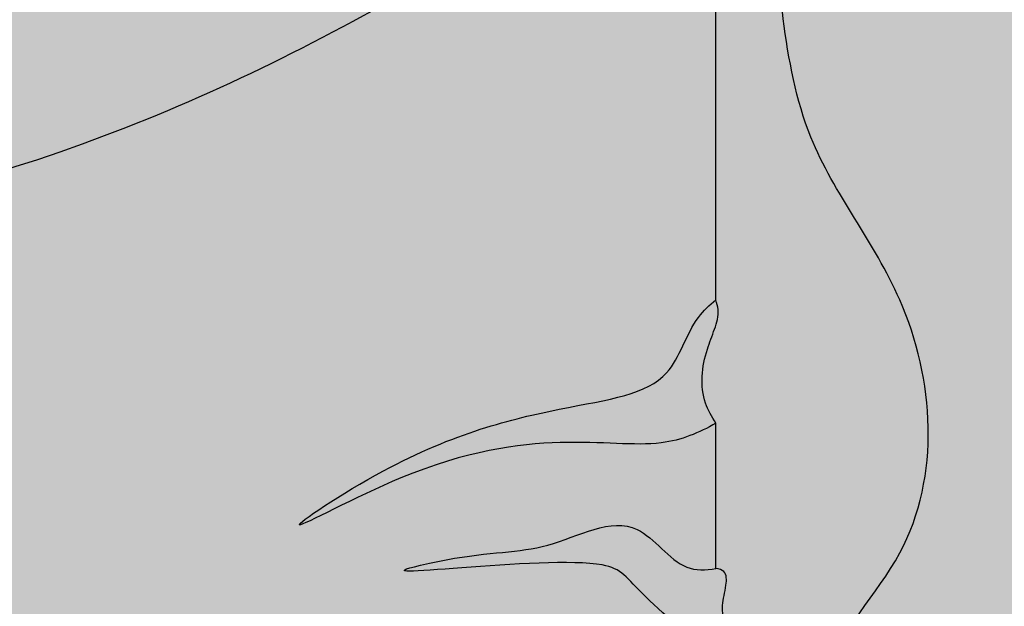
# Model space of a CAD drawing. Units: inches. Extents: x 1704 to 6393, y -157 to 1172.
# Tile 34 of 122: x 2548.79 to 2563.15, y 139.14 to 147.7. Entities that reach past the tile are written whole.
import ezdxf

# ---------------------------------------------------------------- set-up
doc = ezdxf.new("R2010")
doc.units = ezdxf.units.IN
doc.header["$MEASUREMENT"] = 0
for name, color, linetype, lineweight in [('A-ANNO-DIMS', 7, 'Continuous', 13), ('A-FURN', 8, 'Continuous', 18), ('estofado', 7, 'Continuous', 25)]:
    doc.layers.add(name, color=color, linetype=linetype, lineweight=lineweight)
doc.layers.add('A-FLOR-PATT', color=7, linetype='Continuous', lineweight=13, true_color=0xf2f2f2)
doc.styles.get("Standard").update_dxf_attribs({"font": 'arial.ttf'})
doc.dimstyles.get("Standard").update_dxf_attribs({"dimtxt": 6, "dimasz": 2, "dimexe": 0.18, "dimexo": 0.0625, "dimgap": 0.09, "dimtad": 0, "dimtih": 1, "dimtoh": 1, "dimdec": 1, "dimzin": 0, "dimdsep": 46, "dimlunit": 3, "dimtxsty": 'Standard', "dimblk": 'ARCHTICK', "dimcen": 0.09, "dimadec": 0, "dimazin": 0, "dimtfac": 1, "dimtdec": 1, "dimtofl": 0, "dimtmove": 0, "dimatfit": 3, "dimfxl": 1, "dimtolj": 1, "dimtzin": 0, "dimarcsym": 0})

# ---------------------------------------------------------------- blocks, each defined once
blk = doc.blocks.new('Cama Box Regencia LOLA')
at = {"layer": 'estofado', "ltscale": 0.2}
h = blk.add_hatch(color=256, dxfattribs=at)
h.dxf.hatch_style = 1
h.set_gradient(color1=(240, 232, 219), color2=(213, 190, 154), one_color=1, tint=0.7200000286102295)
edge = h.paths.add_edge_path()
edge.add_line((-0.8000000000000682, -0.1548023628405417), (-0.863597199697665, -0.2293271111754507))
edge.add_spline(control_points=[(-0.8635971996977787, -0.2293271111754507), (-0.8537222782123308, -0.258285373872468), (-0.8269013755602826, -0.3369378214810581), (-0.8674912876567759, -0.4595932758330151), (-0.8253488717912205, -0.6001498518888299), (-0.8771423076391329, -0.7139760714239288), (-0.8243323781925938, -0.8129899320257435), (-0.885044987287756, -0.8716602542656914), (-0.879518062107536, -0.9542863467743244), (-0.8339551707063037, -1.008464155856984), (-0.8245672924600739, -1.059984630119799), (-0.8208601923470268, -1.104655887174089), (-0.8073908324747662, -1.131238421004809), (-0.7999999999999546, -1.145824641594799)], knot_values=[0, 0, 0, 0, 0.0901802310564388, 0.2449351320798513, 0.3646438241986237, 0.5132330690395209, 0.5950634960661151, 0.646820388242338, 0.740988272125753, 0.8098674202588053, 0.8551784313864677, 0.8950360916221496, 0.9434986994854018, 0.9434986994854018, 0.9434986994854018, 0.9434986994854018], degree=3, periodic=0)
edge.add_line((-0.7999999999999546, -1.145824641594856), (-0.7999999999999546, -0.9571831923306604))
edge.add_spline(control_points=[(-0.8000000000001818, -0.9571831923294098), (-0.8003674620557603, -0.9560020588672273), (-0.8014778173377408, -0.9524330433489467), (-0.799534669348418, -0.9460450666617248), (-0.7963405736333016, -0.9382358308520792), (-0.7944188048602429, -0.9289040147384638), (-0.7953122817383474, -0.9190683391483389), (-0.7985341887020923, -0.9137677522519994), (-0.7999999999999546, -0.911356242470788)], knot_values=[0, 0, 0, 0, 0.0036609130031785, 0.0110621328900358, 0.0190316076023675, 0.0292873612819121, 0.0393286152452009, 0.0477100398955968, 0.0477100398955968, 0.0477100398955968, 0.0477100398955968], degree=3, periodic=0)
edge.add_line((-0.8000000000000682, -0.9113562424705037), (-0.7999999999999546, -0.8573491405791173))
edge.add_spline(control_points=[(-0.7999999999999546, -0.8573491405791173), (-0.8011509914009592, -0.8570771933481751), (-0.804102924754261, -0.8563797336621519), (-0.8039036519178353, -0.8498286502876908), (-0.8010279369466388, -0.8413595542568258), (-0.805623441450507, -0.8302818657685406), (-0.801318481758244, -0.8238273834048186), (-0.7999999999999546, -0.8218505664625013)], knot_values=[0, 0, 0, 0, 0.0032305881034183, 0.0082854491905874, 0.015951437769388, 0.0315866871777379, 0.0384893971878813, 0.0384893971878813, 0.0384893971878813, 0.0384893971878813], degree=3, periodic=0)
edge.add_line((-0.7999999999999546, -0.821850566462558), (-0.7999999999999546, -0.7800193173444541))
edge.add_spline(control_points=[(-0.7999999999999546, -0.7800193173443404), (-0.7985416092056994, -0.7788853679199974), (-0.7956241855360986, -0.7766169698310819), (-0.7929439183725436, -0.7707329795046576), (-0.7969680334608711, -0.7644035258254576), (-0.7912681985083055, -0.7566015403456845), (-0.7963938877088595, -0.7483952775559715), (-0.798936373489596, -0.7431699116222604), (-0.799999999999841, -0.7409839258539251)], knot_values=[0, 0, 0, 0, 0.0055481279082489, 0.0110986984731684, 0.0174746050947868, 0.0251556172852474, 0.035519246289823, 0.0429729849735991, 0.0429729849735991, 0.0429729849735991, 0.0429729849735991], degree=3, periodic=0)
edge.add_line((-0.7999999999999546, -0.740983925853584), (-0.8000000000000682, -0.1548023628405417))
h = blk.add_hatch(color=256, dxfattribs=at)
h.dxf.hatch_style = 1
h.set_gradient(color1=(240, 232, 219), color2=(213, 190, 154), one_color=1, tint=0.7200000286102295, name='CURVED')
edge = h.paths.add_edge_path()
edge.add_spline(control_points=[(0.343533776195045, -0.8455058148597345), (0.2879313990920309, -0.8167160606696484), (0.2054770794474052, -0.7744470032542381), (0.0954193394759386, -0.7742416952675626), (-0.0885363502328574, -0.7276964167006668), (0.2428192566063672, -0.7672518992321216), (0.345087521536243, -0.8076697826234067), (0.3825206986321063, -0.8228555492498799)], knot_values=[0.0056315103357428, 0.0056315103357428, 0.0056315103357428, 0.0056315103357428, 0.1860138916206105, 0.2660015162584448, 0.3570871810327863, 0.5963901805690979, 0.739731738908988, 0.739731738908988, 0.739731738908988, 0.739731738908988], degree=3, periodic=0)
edge.add_spline(control_points=[(0.3825206986325611, -0.8228555492497662), (0.3974221570828149, -0.8135511441712424), (0.4121061736600496, -0.8037181558521524), (0.4266849906532571, -0.7937075488799225)], knot_values=[1.358237767273279, 1.358237767273279, 1.358237767273279, 1.358237767273279, 1.409915662372559, 1.409915662372559, 1.409915662372559, 1.409915662372559], degree=3, periodic=0)
edge.add_spline(control_points=[(0.4266849905698109, -0.7937075489369932), (0.3998777739682282, -0.7821381809783361), (0.3476761897024971, -0.7634757898491671), (0.2670618099601825, -0.7565375622627358), (0.0835725072796549, -0.7192994417154637), (0.288524529784695, -0.7446405493717521), (0.4247448861246994, -0.7759943071475277), (0.4449816270193879, -0.7810438091316882)], knot_values=[0.1043639306803623, 0.1043639306803623, 0.1043639306803623, 0.1043639306803623, 0.1896363068641149, 0.2696239315019491, 0.3607095962762907, 0.6000125958126024, 0.6446217338078729, 0.6446217338078729, 0.6446217338078729, 0.6446217338078729], degree=3, periodic=0)
edge.add_spline(control_points=[(0.4449816270197289, -0.7810438091316882), (0.5029779388527232, -0.7406836481117695), (0.5966687145296419, -0.6736247633211292), (0.7071737530245628, -0.6656573253703187), (0.7517012483331201, -0.6672238302253392)], knot_values=[1.43159032281798, 1.43159032281798, 1.43159032281798, 1.43159032281798, 1.63814180148235, 1.770695287284994, 1.770695287284994, 1.770695287284994, 1.770695287284994], degree=3, periodic=0)
edge.add_arc((0.7481853615017826, -0.767162003811734), 0.0999999999999888, 58.7920033978138, 87.98512997550938, ccw=False)
edge.add_line((0.8000000000000682, -0.6816328085782289), (0.8000000000000682, -0.154802362840428))
edge.add_line((0.8000000000000682, -0.154802362840428), (-0.7999999999999546, -0.154802362840428))
edge.add_line((-0.7999999999999546, -0.154802362840428), (-0.8000000000000682, -0.7409839258539819))
edge.add_spline(control_points=[(-0.799999999999841, -0.7409839258539251), (-0.7846451382113174, -0.74846387981205), (-0.7568940913494089, -0.7651582159765554), (-0.7559936909002545, -0.8096905380045313), (-0.7049413305308008, -0.8142555457367848), (-0.7013836936888538, -0.8139988647640733)], knot_values=[0.0122267587020837, 0.0122267587020837, 0.0122267587020837, 0.0122267587020837, 0.0594720782072034, 0.1062176618094138, 0.134458043575382, 0.134458043575382, 0.134458043575382, 0.134458043575382], degree=3, periodic=0)
edge.add_spline(control_points=[(-0.7013836936890812, -0.8139988647637892), (-0.6428309483887916, -0.8132695376718857), (-0.532520673001045, -0.8118955240036598), (-0.2390712668254764, -0.6717984706609172), (-0.3892411364554391, -0.7557901092520752), (-0.4591093260188473, -0.8070101468627512), (-0.5571511178645779, -0.795652750469742), (-0.608497950975675, -0.8409486634728295), (-0.6632498050151981, -0.8266781836207997), (-0.6991149398675134, -0.8254126024436914), (-0.719552182989446, -0.8246914287938125)], knot_values=[0, 0, 0, 0, 0.2187005959148062, 0.4120203559900679, 0.4786136596093368, 0.6046444033330721, 0.6969970394608519, 0.7456449795902803, 0.7925683322559657, 0.8547274388453192, 0.8547274388453192, 0.8547274388453192, 0.8547274388453192], degree=3, periodic=0)
edge.add_spline(control_points=[(-0.7195521829781911, -0.824691428792164), (-0.7293124663336812, -0.8248308281530967), (-0.7545977292818407, -0.8216412233076653), (-0.7742556984202338, -0.794819860189591), (-0.7939222919129634, -0.7820064600295497), (-0.799999999999841, -0.7800193173443404)], knot_values=[0.1564883932805935, 0.1564883932805935, 0.1564883932805935, 0.1564883932805935, 0.184397548386913, 0.2313764834161266, 0.2505984550882281, 0.2505984550882281, 0.2505984550882281, 0.2505984550882281], degree=3, periodic=0)
edge.add_line((-0.8000000000000682, -0.7800193173444541), (-0.7999999999999546, -0.8218505664627286))
edge.add_spline(control_points=[(-0.7999999999999546, -0.8218505664625013), (-0.7938082505512511, -0.8290217081292894), (-0.7673857405620766, -0.8512914803976059), (-0.7619109683460011, -0.8661369353891359), (-0.6555700939965164, -0.8510070218793543), (-0.7139793977868294, -0.8637526923380391), (-0.7379026254519659, -0.8623504601624176), (-0.7688129786438367, -0.8813042143888196), (-0.7854260296310259, -0.8561610219318254), (-0.7961930533253962, -0.8566031243811949), (-0.7999999999999546, -0.8573491405791173)], knot_values=[0.0595743221876141, 0.0595743221876141, 0.0595743221876141, 0.0595743221876141, 0.08075289116965, 0.1037414994169835, 0.1697200936249022, 0.1760361327243865, 0.2071371586311508, 0.2404744334261798, 0.2623408547027293, 0.2736604507987723, 0.2736604507987723, 0.2736604507987723, 0.2736604507987723], degree=3, periodic=0)
edge.add_line((-0.7999999999999546, -0.8573491405791173), (-0.8000000000000682, -0.9113562424721521))
edge.add_spline(control_points=[(-0.8000000000000682, -0.9113562424720385), (-0.7937204054647964, -0.9077594990848183), (-0.7710343135782978, -0.8978798065321029), (-0.7213062468074442, -0.9144666877443228), (-0.6268586829058905, -0.862430497409548), (-0.6896594748232019, -0.9045634991654196), (-0.7483442493064559, -0.9189273406958591), (-0.7835301183422417, -0.922920432793262), (-0.7896301351460125, -0.9477657000142585), (-0.7975786973822779, -0.955260590410262), (-0.8000000000001818, -0.9571831923294098)], knot_values=[0.0138560263374175, 0.0138560263374175, 0.0138560263374175, 0.0138560263374175, 0.0348737775836104, 0.0888666909546002, 0.1078792274429341, 0.1267378491223226, 0.1587140219647659, 0.1937574699451985, 0.2174867851300671, 0.2267221218327879, 0.2267221218327879, 0.2267221218327879, 0.2267221218327879], degree=3, periodic=0)
edge.add_line((-0.7999999999999546, -0.957183192329296), (-0.7999999999999546, -1.145824641594742))
edge.add_spline(control_points=[(-0.8000000000002955, -1.145824641594913), (-0.7271039467997298, -1.094596787649038), (-0.4885706936571524, -0.9465888221489535), (-0.0701640902225336, -0.9707493165000187), (0.237911901821235, -0.902164522332157), (0.3435337762145991, -0.845505814843193)], knot_values=[0.1168958193629841, 0.1168958193629841, 0.1168958193629841, 0.1168958193629841, 0.3797203297758731, 0.9577018633805092, 1.31379338443587, 1.31379338443587, 1.31379338443587, 1.31379338443587], degree=3, periodic=0)
h.paths.add_polyline_path([(-0.6766340706021765, -0.6101327540145576, -0.3575266660906883), (-0.7312746368313583, -0.6354535276154252, -0.3575266660894137), (-0.7059538632299791, -0.5808129613865844, -0.1647847126465284), (-0.7059538632300928, -0.2676124402649407, -0.3575266660890756), (-0.7312746368312446, -0.2129718740360431, -0.3575266660908716), (-0.6766340706020629, -0.2382926476369676, -0.0925607043966334), (-0.1295169377724505, -0.2382926476369107, -0.3575266660898965), (-0.0748763715433825, -0.2129718740360431, -0.3575266660894428), (-0.1001971451446479, -0.2676124402649407, -0.1647847126465285), (-0.1001971451445343, -0.5808129613865844, -0.3575266660890756), (-0.0748763715433825, -0.6354535276154821, -0.3575266660898962), (-0.1295169377724505, -0.6101327540146145, -0.0925607043966531)], flags=16)
h.paths.add_polyline_path([(0.0748763715433825, -0.6354535276157094, -0.3575266660910266), (0.1001971451446479, -0.5808129613865844, -0.1647847126465284), (0.1001971451445343, -0.2676124402649407, -0.3575266660890757), (0.0748763715433825, -0.2129718740360431, -0.3575266660898962), (0.1295169377724505, -0.2382926476369107, -0.0925607043966334), (0.6766340706020629, -0.2382926476369676, -0.3575266660908718), (0.7312746368312446, -0.2129718740360431, -0.3575266660894425), (0.7059538632299791, -0.2676124402649407, -0.1647847126465283), (0.7059538632300928, -0.5808129613865844, -0.3575266660890756), (0.7312746368312446, -0.6354535276154821, -0.3575266660908716), (0.6766340706020629, -0.6101327540145576, -0.0925607043966335), (0.1295169377724505, -0.6101327540146145, -0.3575266660906303)], flags=16)
h = blk.add_hatch(color=256, dxfattribs=at)
h.dxf.hatch_style = 1
h.set_gradient(color1=(206, 178, 131), color2=(227, 212, 186), one_color=1, tint=0.8100000023841857, name='CYLINDER')
edge = h.paths.add_edge_path()
edge.add_arc((0.7481853614966667, -0.7671620038115634), 0.0999999999999888, 342.0511336145294, 447.9851299725766)
edge.add_spline(control_points=[(0.7517012483331201, -0.6672238302253392), (0.7071737530245628, -0.6656573253703187), (0.5966687145298692, -0.6736247633211292), (0.5029779388527232, -0.7406836481117125), (0.4449816270195015, -0.7810438091316314)], knot_values=[1.431590322817835, 1.431590322817835, 1.431590322817835, 1.431590322817835, 1.564143808620479, 1.770695287284994, 1.770695287284994, 1.770695287284994, 1.770695287284994], degree=3, periodic=0)
edge.add_spline(control_points=[(0.4449816270195015, -0.7810438091316314), (0.4388957332065502, -0.7852790380018178), (0.4327996148541616, -0.7895089160493285), (0.4266849906533708, -0.7937075488798087)], knot_values=[1.409915662372814, 1.409915662372814, 1.409915662372814, 1.409915662372814, 1.431590322817835, 1.431590322817835, 1.431590322817835, 1.431590322817835], degree=3, periodic=0)
edge.add_spline(control_points=[(0.4266849906533708, -0.7937075488798087), (0.4121061736600496, -0.8037181558521524), (0.3974221570825875, -0.8135511441712991), (0.38252069863222, -0.8228555492498799)], knot_values=[1.358237767273037, 1.358237767273037, 1.358237767273037, 1.358237767273037, 1.409915662372815, 1.409915662372815, 1.409915662372815, 1.409915662372815], degree=3, periodic=0)
edge.add_line((0.3825206986330158, -0.8228555492493114), (0.343533776286904, -0.8455058148063584))
edge.add_spline(control_points=[(0.3435337761924302, -0.8455058148550165), (0.2379119018048641, -0.902164522335795), (-0.0701640902311738, -0.9707493164995071), (-0.4885706936571524, -0.9465888221488967), (-0.7271039467997298, -1.094596787649038), (-0.8000000000000682, -1.145824641594742)], knot_values=[0.1168958193630798, 0.1168958193630798, 0.1168958193630798, 0.1168958193630798, 0.472987340393773, 1.050968873998409, 1.313793384411202, 1.313793384411202, 1.313793384411202, 1.313793384411202], degree=3, periodic=0)
edge.add_spline(control_points=[(-0.8000000000000682, -1.145824641594742), (-0.8038896190357718, -1.14855807951244), (-0.8077744942224853, -1.151305646504738), (-0.8116551946761774, -1.154065647517199)], knot_values=[0.1028719158199011, 0.1028719158199011, 0.1028719158199011, 0.1028719158199011, 0.1168958193630799, 0.1168958193630799, 0.1168958193630799, 0.1168958193630799], degree=3, periodic=0)
edge.add_arc((-0.7536973518524519, -1.235557294053705), 0.1000000000000352, 125.4208969883762, 169.6981795679068)
edge.add_spline(control_points=[(-0.852085287466366, -1.217673946333093), (-0.8521399740518518, -1.217974812833915), (-0.8565649010855622, -1.242328483616745), (-0.8662697220019026, -1.297321141147904), (-0.8487158298532904, -1.34896742172242), (-0.8348745804664758, -1.381844109035796)], knot_values=[0.3128349436863077, 0.3128349436863077, 0.3128349436863077, 0.3128349436863077, 0.3137509534211996, 0.386958004641742, 0.4759027329026081, 0.4759027329026081, 0.4759027329026081, 0.4759027329026081], degree=3, periodic=0)
edge.add_spline(control_points=[(-0.8348745804664758, -1.38184410903591), (-0.8226532004149476, -1.367823298399059), (-0.8056354908857201, -1.352141651537124), (-0.7460155199962628, -1.32170802000337)], knot_values=[0.0062456970656236, 0.0062456970656236, 0.0062456970656236, 0.0062456970656236, 0.0554759259147193, 0.0554759259147193, 0.0554759259147193, 0.0554759259147193], degree=3, periodic=0)
edge.add_spline(control_points=[(-0.7460155200169539, -1.321708019985464), (-0.6188339616464873, -1.25080943574278), (-0.3488365122128698, -1.179158668568902), (0.0338148848931041, -1.279726484458706), (0.3977250465933366, -1.412092721352792), (0.6449024721503065, -1.106270719748692), (0.7873766543807506, -1.256744909425322), (0.8547271521993025, -1.327877176513538)], knot_values=[0.0991852523588446, 0.0991852523588446, 0.0991852523588446, 0.0991852523588446, 0.5236467270390676, 0.9270872950244264, 1.289918234564769, 1.564439021262726, 1.810554634340498, 1.810554634340498, 1.810554634340498, 1.810554634340498], degree=3, periodic=0)
edge.add_arc((0.5509678495186563, -1.223443291813453), 0.3212104454069235, 341.0267878798241, 383.7782184284114)
edge.add_arc((1.292676354991499, -0.9435407756057543), 0.4723459732861395, 162.0511336103901, 198.5657216587827, ccw=False)
h = blk.add_hatch(color=256, dxfattribs=at)
h.dxf.hatch_style = 1
h.set_gradient(color1=(240, 232, 219), color2=(137, 106, 57), one_color=1, tint=0.3799999952316284, name='CURVED')
edge = h.paths.add_edge_path()
edge.add_spline(control_points=[(-0.7999999999999546, -0.8573491405791173), (-0.7961930533253962, -0.8566031243811949), (-0.7854260296310259, -0.8561610219318254), (-0.7688129786438367, -0.8813042143888196), (-0.7379026254519659, -0.8623504601624176), (-0.7139793977868294, -0.8637526923380391), (-0.6555700939965164, -0.8510070218793543), (-0.7619109683460011, -0.8661369353891359), (-0.7673857405620766, -0.8512914803976059), (-0.7938082505512511, -0.8290217081292894), (-0.7999999999999546, -0.8218505664625013)], knot_values=[0.0595743221876141, 0.0595743221876141, 0.0595743221876141, 0.0595743221876141, 0.0708939182836571, 0.0927603395602066, 0.1260976143552356, 0.1571986402619999, 0.1635146793614841, 0.2294932735694029, 0.2524818818167364, 0.2736604507987723, 0.2736604507987723, 0.2736604507987723, 0.2736604507987723], degree=3, periodic=0)
edge.add_spline(control_points=[(-0.7999999999999546, -0.8218505664625013), (-0.801318481758244, -0.8238273834048186), (-0.805623441450507, -0.8302818657685406), (-0.8010279369466388, -0.8413595542568258), (-0.8039036519178353, -0.8498286502876908), (-0.804102924754261, -0.8563797336621519), (-0.8011509914009592, -0.8570771933481751), (-0.7999999999999546, -0.8573491405791173)], knot_values=[0, 0, 0, 0, 0.0069027100101435, 0.0225379594184934, 0.030203947997294, 0.0352588090844631, 0.0384893971878813, 0.0384893971878813, 0.0384893971878813, 0.0384893971878813], degree=3, periodic=0)
h = blk.add_hatch(color=256, dxfattribs=at)
h.dxf.hatch_style = 1
h.set_gradient(color1=(240, 232, 219), color2=(137, 106, 57), one_color=1, tint=0.3799999952316284, name='CURVED')
edge = h.paths.add_edge_path()
edge.add_spline(control_points=[(-0.8000000000001818, -0.9571831923294098), (-0.7975786973822779, -0.955260590410262), (-0.7896301351460125, -0.9477657000142585), (-0.7835301183422417, -0.922920432793262), (-0.7483442493064559, -0.9189273406958591), (-0.6896594748232019, -0.9045634991654196), (-0.6268586829058905, -0.862430497409548), (-0.7213062468074442, -0.9144666877443228), (-0.7710343135782978, -0.8978798065321029), (-0.7937204054647964, -0.9077594990848183), (-0.8000000000000682, -0.9113562424720385)], knot_values=[0.0138560263374175, 0.0138560263374175, 0.0138560263374175, 0.0138560263374175, 0.0230913630401383, 0.0468206782250069, 0.0818641262054395, 0.1138402990478828, 0.1326989207272713, 0.1517114572156053, 0.205704370586595, 0.2267221218327879, 0.2267221218327879, 0.2267221218327879, 0.2267221218327879], degree=3, periodic=0)
edge.add_spline(control_points=[(-0.7999999999999546, -0.911356242470788), (-0.7985341887020923, -0.9137677522519994), (-0.7953122817383474, -0.9190683391483389), (-0.7944188048602429, -0.9289040147384638), (-0.7963405736333016, -0.9382358308520792), (-0.799534669348418, -0.9460450666617248), (-0.8014778173377408, -0.9524330433489467), (-0.8003674620557603, -0.9560020588672273), (-0.8000000000001818, -0.9571831923294098)], knot_values=[0, 0, 0, 0, 0.008381424650396, 0.0184226786136847, 0.0286784322932294, 0.0366479070055611, 0.0440491268924183, 0.0477100398955968, 0.0477100398955968, 0.0477100398955968, 0.0477100398955968], degree=3, periodic=0)
for points in [[(-0.7999999999999546, -0.8573491405790605), (-0.7999999999999546, -0.9113562424710153)], [(-0.7999999999999546, -0.9571831923292393), (-0.7999999999999546, -1.145824641594799)]]:
    blk.add_lwpolyline(points, dxfattribs=at)
for points, knots in [([(-0.8635971996977787, -0.2293271111754507), (-0.8537222782123597, -0.2582853738724713), (-0.8269013755602529, -0.3369378214810687), (-0.8674912876567628, -0.459593275832977), (-0.8253488717912105, -0.6001498518888299), (-0.8771423076387755, -0.7139760714238776), (-0.824332378192706, -0.8129899320257793), (-0.8850449872876955, -0.8716602542656513), (-0.8795180621076731, -0.9542863467744586), (-0.8339551707061605, -1.008464155856879), (-0.8245672924602526, -1.059984630119836), (-0.820860192346876, -1.104655887174075), (-0.8073908324747767, -1.131238421004865), (-0.7999999999999546, -1.145824641594799)], [0, 0, 0, 0, 0.0901802310564388, 0.2449351320798513, 0.3646438241986237, 0.5132330690395209, 0.5950634960661151, 0.646820388242338, 0.740988272125753, 0.8098674202588053, 0.8551784313864677, 0.8950360916221496, 0.9434986994854018, 0.9434986994854018, 0.9434986994854018, 0.9434986994854018]), ([(-0.7999999999999546, -0.8218505664625013), (-0.8013184817582112, -0.8238273834047737), (-0.8056234414505565, -0.8302818657685486), (-0.8010279369466333, -0.8413595542568746), (-0.8039036519179351, -0.8498286502876482), (-0.80410292475424, -0.8563797336621606), (-0.8011509914010776, -0.857077193348196), (-0.7999999999999546, -0.8573491405791173)], [0, 0, 0, 0, 0.0069027100101435, 0.0225379594184934, 0.030203947997294, 0.0352588090844631, 0.0384893971878813, 0.0384893971878813, 0.0384893971878813, 0.0384893971878813]), ([(-0.7999999999999546, -0.8218505664625013), (-0.7938082505512511, -0.8290217081292894), (-0.7673857405620766, -0.8512914803976059), (-0.7619109683460011, -0.8661369353891359), (-0.6555700939965164, -0.8510070218793543), (-0.7139793977868294, -0.8637526923380391), (-0.7379026254519659, -0.8623504601624176), (-0.7688129786438367, -0.8813042143888196), (-0.7854260296310259, -0.8561610219318254), (-0.7961930533253962, -0.8566031243811949), (-0.7999999999999546, -0.8573491405791173)], [0.0595743221876141, 0.0595743221876141, 0.0595743221876141, 0.0595743221876141, 0.08075289116965, 0.1037414994169835, 0.1697200936249022, 0.1760361327243865, 0.2071371586311508, 0.2404744334261798, 0.2623408547027293, 0.2736604507987723, 0.2736604507987723, 0.2736604507987723, 0.2736604507987723]), ([(-0.8116551946761774, -1.154065647517199), (-0.7350455857787211, -1.099579968801037), (-0.493473113061782, -0.9463057365681493), (-0.0701640902311738, -0.9707493164995071), (0.2379119018048641, -0.902164522335795), (0.3435337761924302, -0.8455058148550165)], [0.1028719158199011, 0.1028719158199011, 0.1028719158199011, 0.1028719158199011, 0.3797203297758731, 0.9577018633805092, 1.313793384411202, 1.313793384411202, 1.313793384411202, 1.313793384411202]), ([(-0.8000000000000682, -0.9113562424720385), (-0.7937204054647964, -0.9077594990848183), (-0.7710343135782978, -0.8978798065321029), (-0.7213062468074442, -0.9144666877443228), (-0.6268586829058905, -0.862430497409548), (-0.6896594748232019, -0.9045634991654196), (-0.7483442493064559, -0.9189273406958591), (-0.7835301183422417, -0.922920432793262), (-0.7896301351460125, -0.9477657000142585), (-0.7975786973822779, -0.955260590410262), (-0.8000000000001818, -0.9571831923294098)], [0.0138560263374175, 0.0138560263374175, 0.0138560263374175, 0.0138560263374175, 0.0348737775836104, 0.0888666909546002, 0.1078792274429341, 0.1267378491223226, 0.1587140219647659, 0.1937574699451985, 0.2174867851300671, 0.2267221218327879, 0.2267221218327879, 0.2267221218327879, 0.2267221218327879]), ([(-0.7999999999999546, -0.911356242470788), (-0.7985341887021342, -0.913767752252043), (-0.795312281738289, -0.9190683391482961), (-0.7944188048601522, -0.9289040147384582), (-0.7963405736334027, -0.9382358308520572), (-0.7995346693483358, -0.946045066661701), (-0.8014778173378848, -0.9524330433489994), (-0.800367462055735, -0.9560020588672482), (-0.8000000000001818, -0.9571831923294098)], [0, 0, 0, 0, 0.008381424650396, 0.0184226786136847, 0.0286784322932294, 0.0366479070055611, 0.0440491268924183, 0.0477100398955968, 0.0477100398955968, 0.0477100398955968, 0.0477100398955968])]:
    blk.add_open_spline(points, degree=3, knots=knots, dxfattribs=at)
blk = doc.blocks.new('_ArchTick')
at = {"color": 0, "linetype": 'ByBlock', "const_width": 0.15}
blk.add_lwpolyline([(-0.5, -0.5), (0.5, 0.5)], dxfattribs=at)
blk = doc.blocks.new('*D93')
at = {"layer": 'A-ANNO-DIMS', "color": 0, "lineweight": -2, "transparency": 16777216}
for p, q in [((2605.286074000001, 895.2129740000005), (1829.697551000002, 895.2129740000003)), ((1829.877551000002, 895.2129740000003), (1829.877551000002, 495.8664119263302)), ((1829.877551000002, 90.2129739999999), (1829.877551000002, 489.5595360736699)), ((2605.286074000001, 90.21297400000003), (1829.697551000002, 90.2129739999999))]:
    blk.add_line(p, q, dxfattribs=at)
at = {"layer": 'Defpoints', "color": 0, "lineweight": -3, "transparency": 16777216}
for p in [(2605.348574000001, 895.2129740000005), (1829.877551000002, 90.2129739999999), (2605.348574000001, 90.21297400000003)]:
    blk.add_point(p, dxfattribs=at)
at = {"layer": 'A-ANNO-DIMS', "color": 0, "lineweight": -2, "transparency": 16777216, "xscale": 2, "yscale": 2, "zscale": 2}
for p, rotation in [((1829.877551000002, 895.2129740000003), 90), ((1829.877551000002, 90.2129739999999), 270)]:
    blk.add_blockref('_ArchTick', p, dxfattribs=dict(at, rotation=rotation))
at = {"layer": 'A-ANNO-DIMS', "color": 0, "transparency": 16777216, "insert": (1829.877551000001, 492.7129739999994), "char_height": 6, "attachment_point": 5}
blk.add_mtext('\\A1;805', dxfattribs=at)

msp = doc.modelspace()

# ---------------------------------------------------------------- hatches: boundary and pattern name
at = {"layer": 'A-FLOR-PATT', "transparency": 33554528}
h = msp.add_hatch(color=256, dxfattribs=at)
h.dxf.hatch_style = 1
h.paths.add_polyline_path([(2325.348574056059, 863.2129735309796), (2325.348574056059, 887.2129735309796), (2263.348574056059, 887.2129735309796), (2167.348574056059, 887.2129735309794), (2081.348574056061, 887.2129735309792), (2081.348574056061, 719.2129735309785), (2277.348574056059, 719.2129735309787), (2277.348574056059, 711.2129735309788), (2277.348574056059, 372.212973530979), (2349.348574056059, 372.212973530979), (2381.348574056059, 372.2129735309789), (2381.348574056059, 364.2129735309789), (2353.348574056059, 364.2129735309789), (2353.348574056059, 270.2129735309788), (2381.348574056059, 270.2129735309788), (2381.348574056059, 266.2129735309788), (2357.348574056059, 266.2129735309788), (2357.348574056059, 98.21297353097884), (2381.348574056059, 98.21297353097897), (2385.181056550604, 98.21297353097884), (2386.482186711948, 98.21297353097884), (2424.21496140017, 98.21297353097884), (2425.516091561514, 98.21297353097884), (2429.348574056059, 98.21297353097897), (2597.348574056059, 98.21297353097884), (2597.348574056059, 146.2129735309788), (2597.348574056059, 218.2129735309788), (2597.348574056059, 266.2129735309788), (2423.348574056059, 266.2129735309788), (2423.348574056059, 270.2129735309788), (2473.348574056059, 270.2129735309788), (2473.348574056059, 294.2129735309789), (2477.348574056059, 294.2129735309789), (2477.348574056059, 270.2129735309788), (2547.348574056059, 270.2129735309788), (2547.348574056059, 364.2129735309788), (2477.348574056059, 364.2129735309788), (2477.348574056059, 318.2129735309788), (2473.348574056059, 318.2129735309787), (2473.348574056059, 364.2129735309789), (2423.348574056059, 364.2129735309788), (2423.348574056059, 372.2129735309788), (2469.348574056059, 372.2129735309788), (2469.348574056059, 459.2129735309789), (2469.348574056059, 538.2129735309788), (2350.348574056059, 538.2129735309788), (2350.348574056059, 565.7129735309788), (2358.348574056059, 565.7129735309788), (2358.348574056059, 545.2129735309788), (2420.348574056059, 545.2129735309788), (2420.348574056059, 610.2129735309788), (2358.348574056059, 610.2129735309788), (2358.348574056059, 589.7129735309788), (2350.348574056059, 589.7129735309788), (2350.348574056059, 615.2129735309788), (2425.348574056059, 615.2129735309788), (2425.348574056059, 607.2129735309788), (2425.348574056059, 546.2129735309788), (2469.348574056059, 546.2129735309788), (2514.34857405606, 546.212973530979), (2514.34857405606, 607.2129735309788), (2449.348574056059, 607.2129735309788), (2449.348574056059, 615.2129735309788), (2451.737974987759, 615.2129735309788), (2451.737974987759, 659.2129735309788), (2427.737974987759, 659.2129735309788), (2427.737974987759, 665.2129735309788), (2367.737974987758, 665.2129735309788), (2367.737974987758, 667.2129735309788), (2367.737974987758, 711.2129735309788), (2325.348574056059, 711.2129735309788), (2325.348574056059, 719.2129735309785), (2325.348574056059, 755.2129735309787), (2325.348574056059, 763.2129735309788)])
h.paths.add_polyline_path([(2233.85817000392, 822.532660166629, -0.1872470486944155), (2233.85817000392, 809.1396667958562), (2231.697030374885, 808.8044951349628, 0.0848927708004382), (2233.130501812631, 814.4858417746204), (2230.423974436808, 814.4858417746204, -0.1042581087707907), (2228.553363812687, 808.3129425443484), (2217.750790159711, 807.1555239386723, -0.2222222222222219), (2217.750790159711, 824.5168030238124), (2228.553363812687, 823.3593844181363, -0.1042581087707933), (2230.423974436808, 817.1864851878643), (2233.130501812631, 817.1864851878643, 0.08489277080044), (2231.697030374885, 822.8678318275219)], flags=16)
h.paths.add_polyline_path([(2213.621360876743, 833.1974425663823), (2213.621360876743, 798.4748843961024), (2156.047684459484, 798.4748843961034), (2156.047684459485, 833.1974425663813)], flags=16)
h.paths.add_polyline_path([(2203.931929661768, 848.0987249710489), (2205.089348267444, 837.2961513180724, -0.2222222222222264), (2187.728069182304, 837.2961513180724), (2188.88548778798, 848.0987249710485, -0.104258108770792), (2195.058387018252, 849.9693355951691), (2195.058387018252, 852.6758629709927, 0.084892770800438), (2189.377040378595, 851.2423915332469), (2189.712212039488, 853.4035311622828, -0.1872470486944166), (2203.105205410261, 853.4035311622828), (2203.440377071154, 851.2423915332469, 0.084892770800438), (2197.759030431496, 852.6758629709927), (2197.759030431496, 849.9693355951691, -0.1042581087707896)], flags=16)
h.paths.add_polyline_path([(2181.940976153924, 837.2961513180726, -0.2222222222222323), (2164.579697068783, 837.2961513180724), (2165.73711567446, 848.0987249710487, -0.1042581087707905), (2171.910014904732, 849.9693355951691), (2171.910014904732, 852.6758629709927, 0.0848927708004445), (2166.228668265074, 851.2423915332469), (2166.563839925967, 853.403531162283, -0.1872470486944096), (2179.95683329674, 853.4035311622828), (2180.292004957633, 851.2423915332465, 0.0848927708004458), (2174.610658317976, 852.6758629709927), (2174.610658317976, 849.9693355951691, -0.104258108770801), (2180.783557548248, 848.0987249710482)], flags=16)
h.paths.add_polyline_path([(2205.089348267444, 794.376175644412), (2203.931929661768, 783.5736019914364, -0.1042581087707934), (2197.759030431496, 781.7029913673155), (2197.759030431496, 778.9964639914921, 0.084892770800439), (2203.440377071154, 780.4299354292382), (2203.105205410261, 778.2687958002022, -0.1872470486944172), (2189.712212039488, 778.2687958002018), (2189.377040378595, 780.4299354292377, 0.0848927708004369), (2195.058387018252, 778.9964639914919), (2195.058387018252, 781.7029913673153, -0.1042581087707904), (2188.88548778798, 783.5736019914358), (2187.728069182304, 794.3761756444126, -0.2222222222222231)], flags=16)
h.paths.add_polyline_path([(2181.940976153924, 794.376175644412), (2180.783557548248, 783.5736019914364, -0.1042581087708008), (2174.610658317976, 781.7029913673153), (2174.610658317976, 778.9964639914921, 0.0848927708004458), (2180.292004957633, 780.4299354292382), (2179.95683329674, 778.268795800202, -0.1872470486944096), (2166.563839925967, 778.2687958002018), (2166.228668265074, 780.4299354292378, 0.0848927708004446), (2171.910014904732, 778.9964639914919), (2171.910014904732, 781.7029913673153, -0.1042581087707904), (2165.73711567446, 783.5736019914358), (2164.579697068783, 794.3761756444123, -0.2222222222222294)], flags=16)
h.paths.add_polyline_path([(2151.918255176517, 807.1555239386723), (2141.115681523541, 808.3129425443484, -0.1042581087707911), (2139.24507089942, 814.4858417746204), (2136.538543523597, 814.4858417746204, 0.08489277080044), (2137.972014961343, 808.8044951349626), (2135.810875332307, 809.1396667958562, -0.1872470486944109), (2135.810875332307, 822.5326601666285), (2137.972014961343, 822.8678318275221, 0.0848927708004416), (2136.538543523597, 817.1864851878643), (2139.24507089942, 817.1864851878643, -0.104258108770793), (2141.115681523541, 823.3593844181363), (2151.918255176517, 824.5168030238124, -0.2222222222222205)], flags=16)
h.paths.add_polyline_path([(2357.868011454448, 363.4102250290031), (2358.813881560335, 363.4102250290031, 0.7537604849588476)], flags=16)
h.paths.add_polyline_path([(2372.241054283868, 363.1167008961685), (2372.248110816919, 363.1167008961685), (2372.248110816919, 363.3425764997267), (2371.30224071103, 363.3425764997267), (2371.30224071103, 363.1392706554335, -1.360391292333951)], flags=16)
h.paths.add_polyline_path([(2371.309297244092, 272.7157694655011), (2371.30224071103, 272.7157694655011), (2371.30224071103, 272.4898938619428), (2372.248110816919, 272.4898938619428), (2372.248110816919, 272.6931997062759, -1.360391292393621)], flags=16)
h.paths.add_polyline_path([(2357.875067987504, 272.7157694655011), (2357.868011454452, 272.7157694655011), (2357.868011454452, 272.4898938619428), (2358.813881560341, 272.4898938619428), (2358.813881560341, 272.6931997062361, -1.360391292333948)], flags=16)
h.paths.add_polyline_path([(2353.768696905258, 363.0736921025416), (2376.347425366111, 363.0736921025416), (2376.347425366111, 272.7587782591281), (2353.768696905258, 272.7587782591281)], flags=16)
h.paths.add_polyline_path([(2354.772195947961, 362.0701930598379), (2375.343926323407, 362.0701930598379), (2375.343926323407, 273.7622773018316), (2354.772195947961, 273.7622773018318)], flags=0)
h.paths.add_polyline_path([(2357.868011454452, 363.3425764997267), (2358.813881560341, 363.3425764997266), (2358.813881560341, 363.1167008961684), (2357.868011454452, 363.1167008961684)], flags=16)
h.paths.add_polyline_path([(2359.287941640134, 359.1843485433627), (2359.287941640134, 360.0631949744305), (2370.828180631237, 360.0631949744362), (2370.828180631237, 359.1843485433769), (2374.332057422314, 359.1843485433812), (2374.332057422312, 358.4635369582513), (2372.835178716611, 358.4635369582524), (2372.835178716611, 357.5410357047662), (2374.332057422314, 357.5410357047678), (2374.332057422312, 356.8202241196381), (2372.835178716611, 356.820224119639), (2372.835178716611, 355.897722866153), (2374.332057422314, 355.8977228661546), (2374.332057422312, 355.1769112810248), (2372.835178716611, 355.1769112810259), (2372.835178716611, 354.2544100275397), (2374.332057422334, 354.2544100275415), (2374.332057422331, 353.5335984424117), (2372.835178716631, 353.5335984424126), (2372.835178716631, 352.6110971889265), (2374.332057422334, 352.6110971889282), (2374.332057422331, 351.8902856037984), (2372.835178716631, 351.8902856037993), (2372.835178716631, 350.9677843503132), (2374.332057422334, 350.967784350315), (2374.332057422331, 350.2469727651852), (2372.835178716631, 350.2469727651861), (2372.835178716631, 349.3244715117), (2374.332057422334, 349.3244715117017), (2374.332057422331, 348.603659926572), (2372.835178716631, 348.6036599265729), (2372.835178716631, 347.6811586730868), (2374.332057422334, 347.6811586730886), (2374.332057422331, 346.9603470879587), (2372.835178716631, 346.9603470879598), (2372.835178716631, 346.0378458344735), (2374.332057422334, 346.0378458344753), (2374.332057422331, 345.3170342493456), (2372.835178716631, 345.3170342493465), (2372.835178716631, 344.3945329958605), (2374.332057422334, 344.3945329958621), (2374.332057422331, 343.6737214107324), (2372.835178716631, 343.6737214107334), (2372.835178716631, 342.751220157247), (2374.332057422334, 342.7512201572489), (2374.332057422331, 342.0304085721191), (2372.835178716631, 342.03040857212), (2372.835178716631, 341.1079073186338), (2374.332057422334, 341.1079073186356), (2374.332057422331, 340.3870957335057), (2372.835178716631, 340.3870957335066), (2372.835178716631, 339.4645944800207), (2374.332057422334, 339.4645944800223), (2374.332057422331, 338.7437828948924), (2372.835178716648, 338.7437828948933), (2372.835178716648, 337.8212816414076), (2374.332057422334, 337.8212816414093), (2374.332057422331, 337.1004700562794), (2372.835178716648, 337.1004700562803), (2372.835178716648, 336.1779688027942), (2374.332057422334, 336.1779688027961), (2374.332057422331, 335.4571572176662), (2372.835178716648, 335.4571572176673), (2372.835178716648, 334.5346559641809), (2374.332057422334, 334.5346559641828), (2374.332057422331, 333.8138443790529), (2372.835178716648, 333.8138443790539), (2372.835178716648, 332.8913431255679), (2374.332057422334, 332.8913431255696), (2374.332057422331, 332.1705315404397), (2372.835178716648, 332.1705315404406), (2372.835178716648, 331.2480302869545), (2374.332057422334, 331.2480302869563), (2374.332057422331, 330.5272187018265), (2372.835178716648, 330.5272187018273), (2372.835178716648, 329.6047174483413), (2374.332057422334, 329.6047174483431), (2374.332057422331, 328.8839058632133), (2372.835178716648, 328.8839058632143), (2372.835178716648, 327.9614046097282), (2374.332057422334, 327.9614046097298), (2374.332057422331, 327.2405930246), (2372.835178716648, 327.2405930246009), (2372.835178716648, 326.3180917711149), (2374.332057422334, 326.3180917711167), (2374.332057422331, 325.5972801859869), (2372.835178716648, 325.5972801859877), (2372.835178716648, 324.6747789325016), (2374.332057422334, 324.6747789325034), (2374.332057422331, 323.9539673473736), (2372.835178716648, 323.9539673473746), (2372.835178716648, 323.0314660938884), (2374.332057422334, 323.0314660938901), (2374.332057422331, 322.3106545087603), (2372.835178716648, 322.3106545087613), (2372.835178716648, 321.3881532552753), (2374.332057422334, 321.388153255277), (2374.332057422331, 320.6673416701471), (2372.835178716648, 320.6673416701481), (2372.835178716648, 319.7448404166621), (2374.332057422334, 319.7448404166638), (2374.332057422331, 319.0240288315339), (2372.835178716648, 319.0240288315348), (2372.835178716648, 318.1015275780487), (2374.332057422334, 318.1015275780504), (2374.332057422331, 317.3807159929205), (2372.835178716648, 317.3807159929214), (2372.835178716648, 316.4582147394357), (2374.332057422334, 316.4582147394373), (2374.332057422331, 315.7374031543073), (2372.835178716648, 315.7374031543084), (2372.835178716648, 314.8149019008223), (2374.332057422334, 314.8149019008241), (2374.332057422331, 314.0940903156943), (2372.835178716648, 314.0940903156952), (2372.835178716648, 313.171589062209), (2374.332057422334, 313.1715890622108), (2374.332057422331, 312.450777477081), (2372.835178716648, 312.4507774770819), (2372.835178716648, 311.5282762235959), (2374.332057422334, 311.5282762235977), (2374.332057422331, 310.8074646384678), (2372.835178716648, 310.8074646384687), (2372.835178716648, 309.8849633849827), (2374.332057422334, 309.8849633849844), (2374.332057422331, 309.1641517998546), (2372.835178716648, 309.1641517998555), (2372.835178716648, 308.2416505463693), (2374.332057422334, 308.2416505463712), (2374.332057422331, 307.5208389612412), (2372.835178716648, 307.5208389612421), (2372.835178716648, 306.5983377077562), (2374.332057422334, 306.598337707758), (2374.332057422331, 305.8775261226281), (2372.835178716648, 305.8775261226289), (2372.835178716648, 304.955024869143), (2374.332057422334, 304.9550248691447), (2374.332057422331, 304.2342132840149), (2372.835178716648, 304.2342132840158), (2372.835178716648, 303.3117120305298), (2374.332057422334, 303.3117120305316), (2374.332057422331, 302.5909004454018), (2372.835178716648, 302.5909004454027), (2372.835178716648, 301.6683991919165), (2374.332057422334, 301.6683991919183), (2374.332057422331, 300.9475876067885), (2372.835178716648, 300.9475876067894), (2372.835178716648, 300.0250863533033), (2374.332057422334, 300.025086353305), (2374.332057422331, 299.3042747681752), (2372.835178716648, 299.3042747681761), (2372.835178716648, 298.3817735146902), (2374.332057422334, 298.3817735146919), (2374.332057422331, 297.6609619295621), (2372.835178716648, 297.6609619295629), (2372.835178716648, 296.7384606760769), (2374.332057422334, 296.7384606760786), (2374.332057422331, 296.0176490909488), (2372.835178716648, 296.0176490909498), (2372.835178716648, 295.0951478374636), (2374.332057422334, 295.0951478374653), (2374.332057422331, 294.3743362523355), (2372.835178716648, 294.3743362523364), (2372.835178716648, 293.4518349988504), (2374.332057422334, 293.4518349988522), (2374.332057422331, 292.7310234137224), (2372.835178716648, 292.7310234137233), (2372.835178716648, 291.8085221602371), (2374.332057422334, 291.8085221602389), (2374.332057422331, 291.0877105751091), (2372.835178716648, 291.08771057511), (2372.835178716648, 290.165209321624), (2374.332057422334, 290.1652093216256), (2374.332057422331, 289.4443977364957), (2372.835178716648, 289.4443977364966), (2372.835178716648, 288.5218964830108), (2374.332057422334, 288.5218964830125), (2374.332057422331, 287.8010848978827), (2372.835178716648, 287.8010848978836), (2372.835178716648, 286.8785836443975), (2374.332057422334, 286.8785836443993), (2374.332057422331, 286.1577720592695), (2372.835178716648, 286.1577720592703), (2372.835178716648, 285.2352708057842), (2374.332057422334, 285.2352708057861), (2374.332057422331, 284.5144592206562), (2372.835178716648, 284.514459220657), (2372.835178716648, 283.5919579671712), (2374.332057422334, 283.5919579671728), (2374.332057422331, 282.871146382043), (2372.835178716648, 282.8711463820439), (2372.835178716648, 281.9486451285579), (2374.332057422334, 281.9486451285596), (2374.332057422331, 281.2278335434298), (2372.835178716648, 281.2278335434307), (2372.835178716648, 280.3053322899446), (2374.332057422334, 280.3053322899464), (2374.332057422331, 279.5845207048164), (2372.835178716648, 279.5845207048174), (2372.835178716648, 278.6620194513314), (2374.332057422334, 278.6620194513331), (2374.332057422331, 277.9412078662033), (2372.835178716648, 277.9412078662043), (2372.835178716648, 277.0187066127184), (2374.332057422334, 277.0187066127201), (2374.332057422331, 276.29789502759), (2370.828180631244, 276.2978950275922), (2370.828180631244, 275.7692753872335), (2359.287941640128, 275.7692753872392), (2359.287941640128, 276.2978950275993), (2355.784064849037, 276.2978950276015), (2355.784064849037, 277.0187066126971), (2357.280943554723, 277.0187066126989), (2357.280943554723, 277.9412078662137), (2355.784064849037, 277.9412078662145), (2355.784064849037, 278.6620194513103), (2357.280943554723, 278.6620194513122), (2357.280943554723, 279.5845207048271), (2355.784064849037, 279.584520704828), (2355.784064849037, 280.3053322899236), (2357.280943554723, 280.3053322899253), (2357.280943554723, 281.2278335434403), (2355.784064849037, 281.2278335434412), (2355.784064849037, 281.9486451285369), (2357.280943554723, 281.9486451285387), (2357.280943554723, 282.8711463820535), (2355.784064849037, 282.8711463820543), (2355.784064849037, 283.5919579671501), (2357.280943554723, 283.591957967152), (2357.280943554723, 284.5144592206668), (2355.784064849037, 284.5144592206676), (2355.784064849037, 285.2352708057632), (2357.280943554723, 285.2352708057651), (2357.280943554723, 286.1577720592801), (2355.784064849037, 286.1577720592809), (2355.784064849037, 286.8785836443766), (2357.280943554723, 286.8785836443784), (2357.280943554723, 287.8010848978931), (2355.784064849037, 287.8010848978941), (2355.784064849037, 288.5218964829895), (2357.280943554723, 288.5218964829913), (2357.280943554723, 289.4443977365064), (2355.784064849037, 289.4443977365072), (2355.784064849037, 290.1652093216029), (2357.280943554723, 290.1652093216047), (2357.280943554723, 291.0877105751197), (2355.784064849037, 291.0877105751206), (2355.784064849037, 291.8085221602161), (2357.280943554723, 291.8085221602179), (2357.280943554723, 292.7310234137328), (2355.784064849037, 292.7310234137337), (2355.784064849037, 293.4518349988293), (2357.280943554723, 293.451834998831), (2357.280943554723, 294.3743362523461), (2355.784064849037, 294.3743362523469), (2355.784064849037, 295.0951478374426), (2357.280943554723, 295.0951478374445), (2357.280943554723, 296.0176490909594), (2355.784064849037, 296.0176490909601), (2355.784064849037, 296.7384606760557), (2357.280943554723, 296.7384606760575), (2357.280943554723, 297.6609619295724), (2355.784064849037, 297.6609619295734), (2355.784064849037, 298.3817735146691), (2357.280943554723, 298.3817735146709), (2357.280943554723, 299.3042747681858), (2355.784064849037, 299.3042747681866), (2355.784064849037, 300.0250863532823), (2357.280943554723, 300.0250863532841), (2357.280943554723, 300.9475876067989), (2355.784064849037, 300.9475876067997), (2355.784064849037, 301.6683991918954), (2357.280943554723, 301.6683991918973), (2357.280943554723, 302.5909004454123), (2355.784064849037, 302.5909004454133), (2355.784064849037, 303.3117120305088), (2357.280943554723, 303.3117120305105), (2357.280943554723, 304.2342132840254), (2355.784064849037, 304.2342132840262), (2355.784064849037, 304.9550248691219), (2357.280943554723, 304.9550248691238), (2357.280943554723, 305.8775261226386), (2355.784064849037, 305.8775261226394), (2355.784064849037, 306.5983377077352), (2357.280943554723, 306.5983377077369), (2357.280943554723, 307.5208389612518), (2355.784064849037, 307.5208389612528), (2355.784064849037, 308.2416505463484), (2357.280943554723, 308.2416505463501), (2357.280943554723, 309.1641517998652), (2355.784064849037, 309.1641517998661), (2355.784064849037, 309.8849633849617), (2357.280943554723, 309.8849633849634), (2357.280943554723, 310.8074646384782), (2355.784064849037, 310.8074646384791), (2355.784064849037, 311.5282762235748), (2357.280943554723, 311.5282762235767), (2357.280943554723, 312.4507774770916), (2355.784064849037, 312.4507774770925), (2355.784064849037, 313.171589062188), (2357.280943554723, 313.1715890621898), (2357.280943554723, 314.0940903157049), (2355.784064849037, 314.0940903157058), (2355.784064849037, 314.8149019008013), (2357.280943554723, 314.8149019008032), (2357.280943554723, 315.7374031543179), (2355.784064849037, 315.7374031543187), (2355.784064849037, 316.4582147394146), (2357.280943554723, 316.4582147394165), (2357.280943554723, 317.3807159929311), (2355.784064849037, 317.3807159929321), (2355.784064849037, 318.1015275780277), (2357.280943554723, 318.1015275780295), (2357.280943554723, 319.0240288315445), (2355.784064849037, 319.0240288315454), (2355.784064849037, 319.744840416641), (2357.280943554723, 319.7448404166428), (2357.280943554723, 320.6673416701576), (2355.784064849037, 320.6673416701585), (2355.784064849037, 321.3881532552541), (2357.280943554723, 321.388153255256), (2357.280943554723, 322.3106545087708), (2355.784064849037, 322.3106545087718), (2355.784064849037, 323.0314660938674), (2357.280943554723, 323.0314660938692), (2357.280943554723, 323.9539673473843), (2355.784064849037, 323.9539673473851), (2355.784064849037, 324.6747789324806), (2357.280943554723, 324.6747789324824), (2357.280943554723, 325.5972801859974), (2355.784064849037, 325.5972801859983), (2355.784064849037, 326.3180917710939), (2357.280943554723, 326.3180917710958), (2357.280943554723, 327.2405930246105), (2355.784064849037, 327.2405930246113), (2355.784064849037, 327.9614046097071), (2357.280943554723, 327.961404609709), (2357.280943554723, 328.8839058632238), (2355.784064849037, 328.8839058632245), (2355.784064849037, 329.6047174483202), (2357.280943554723, 329.604717448322), (2357.280943554723, 330.527218701837), (2355.784064849037, 330.5272187018379), (2355.784064849037, 331.2480302869335), (2357.280943554723, 331.2480302869353), (2357.280943554723, 332.1705315404502), (2355.784064849037, 332.170531540451), (2355.784064849037, 332.8913431255468), (2357.280943554723, 332.8913431255486), (2357.280943554723, 333.8138443790634), (2355.784064849037, 333.8138443790642), (2355.784064849037, 334.5346559641599), (2357.280943554723, 334.5346559641618), (2357.280943554723, 335.4571572176767), (2355.784064849037, 335.4571572176776), (2355.784064849037, 336.1779688027732), (2357.280943554723, 336.177968802775), (2357.280943554723, 337.1004700562898), (2355.784064849037, 337.1004700562908), (2355.784064849037, 337.8212816413864), (2357.280943554723, 337.8212816413883), (2357.280943554723, 338.7437828949031), (2355.784064849037, 338.743782894904), (2355.784064849037, 339.4645944799996), (2357.280943554706, 339.4645944800013), (2357.280943554706, 340.3870957335163), (2355.784064849037, 340.3870957335173), (2355.784064849037, 341.1079073186129), (2357.280943554706, 341.1079073186146), (2357.280943554706, 342.0304085721296), (2355.784064849037, 342.0304085721304), (2355.784064849037, 342.7512201572262), (2357.280943554706, 342.751220157228), (2357.280943554706, 343.6737214107429), (2355.784064849037, 343.6737214107437), (2355.784064849037, 344.3945329958394), (2357.280943554706, 344.3945329958412), (2357.280943554706, 345.317034249356), (2355.784064849037, 345.3170342493569), (2355.784064849037, 346.0378458344526), (2357.280943554706, 346.0378458344544), (2357.280943554706, 346.9603470879692), (2355.784064849037, 346.9603470879701), (2355.784064849037, 347.6811586730658), (2357.280943554706, 347.6811586730677), (2357.280943554706, 348.6036599265824), (2355.784064849037, 348.6036599265833), (2355.784064849037, 349.324471511679), (2357.280943554706, 349.3244715116809), (2357.280943554706, 350.2469727651956), (2355.784064849037, 350.2469727651966), (2355.784064849037, 350.9677843502922), (2357.280943554706, 350.9677843502939), (2357.280943554706, 351.8902856038089), (2355.784064849037, 351.8902856038098), (2355.784064849037, 352.6110971889055), (2357.280943554706, 352.6110971889072), (2357.280943554706, 353.5335984424222), (2355.784064849037, 353.533598442423), (2355.784064849037, 354.2544100275187), (2357.280943554686, 354.2544100275204), (2357.280943554686, 355.1769112810354), (2355.784064849017, 355.1769112810362), (2355.784064849017, 355.897722866132), (2357.280943554686, 355.8977228661338), (2357.280943554686, 356.8202241196486), (2355.784064849017, 356.8202241196495), (2355.784064849017, 357.5410357047453), (2357.280943554686, 357.5410357047471), (2357.280943554686, 358.4635369582618), (2355.784064849017, 358.4635369582626), (2355.784064849017, 359.1843485433584)], flags=0)

# ---------------------------------------------------------------- block references
at = {"layer": 'A-FURN', "xscale": 39.22313671019584, "yscale": 39.22313671019584, "zscale": 39.22313671019584, "rotation": 180}
msp.add_blockref('Cama Box Regencia LOLA', (2527.569415053021, 106.0625493409584), dxfattribs=at)

# ---------------------------------------------------------------- dimensions: what is measured, and where the dimension line sits
at = {"layer": 'A-ANNO-DIMS'}
dim = msp.add_linear_dim(base=(1829.877551000002, 90.2129739999999), p1=(2605.348574000001, 895.212974), p2=(2605.348574000001, 90.21297399999999), angle=90, dimstyle='Standard', override={"dimdec": 0, "dimlfac": 1, "dimrnd": 0, "dimzin": 0, "dimdsep": 46, "dimlunit": 2}, dxfattribs=at)
dim.commit()
dim.dimension.update_dxf_attribs({"geometry": '*D93', "text_midpoint": (1829.877551000001, 492.7129739999994)})

doc.saveas('drawing.dxf')
